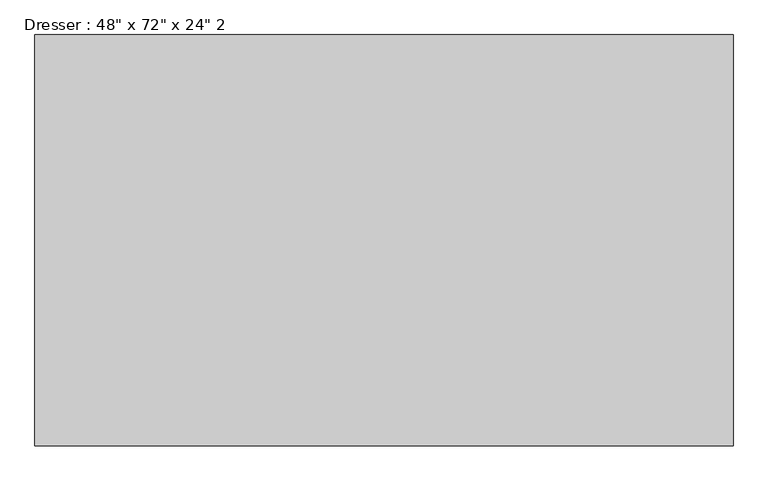
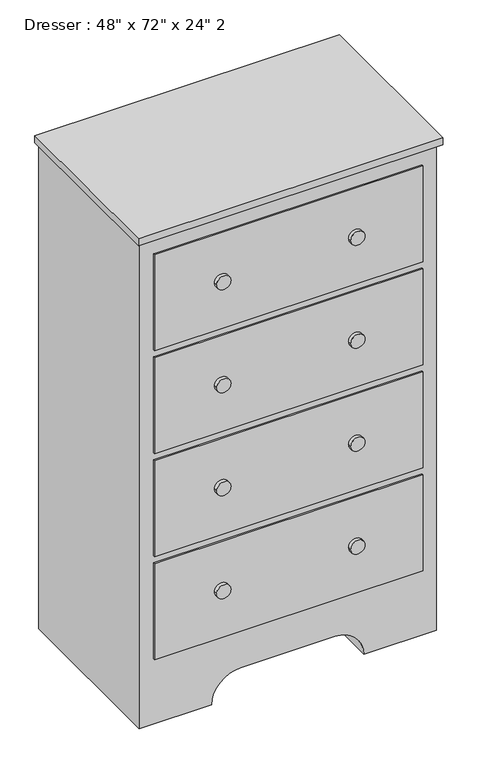
"""IFC4 building model written with IfcOpenShell, lengths in millimetres: furniture geometry."""

from ifc_helpers import new_model, si_unit, point, frame, frame_2d, origin, place, context, project, spatial, polyline, circle_curve, trimmed, segment, composite_curve, outline, extrude, source, transform, mapped, element, save


def furniture_f72bdee3(model_context):
    return source(origin(), model_context, "Body", "SweptSolid", [
        extrude(outline(polyline([(264.2067402, -58.3629541), (264.2067402, -687.0129541), (-802.5932598, -687.0129541), (-802.5932598, -58.3629541), (264.2067402, -58.3629541)])), frame((0.0, 0.0, 1803.4), z_axis=(0.0, 0.0, 1.0), x_axis=(1.0, 0.0, 0.0)), (0.0, 0.0, 1.0), 25.4),
        extrude(outline(composite_curve([segment(polyline([(0.0, 251.5067402), (1803.4, 251.5067402), (1803.4, -789.8932598), (0.0, -789.8932598), (0.0, -535.8932598)]), True, "CONTINUOUS"), segment(trimmed(circle_curve(frame_2d((0.0, -434.2932598)), 101.6), [point((0.0, -535.8932598))], [point((101.6, -434.2932598))], True, "CARTESIAN"), True, "CONTINUOUS"), segment(polyline([(101.6, -434.2932598), (101.6, -104.0932598)]), True, "CONTINUOUS"), segment(trimmed(circle_curve(frame_2d((0.0, -104.0932598)), 101.6), [point((101.6, -104.0932598))], [point((0.0, -2.4932598))], True, "CARTESIAN"), True, "CONTINUOUS"), segment(polyline([(0.0, -2.4932598), (0.0, 251.5067402)]), True, "CONTINUOUS")], self_intersect=False)), frame((0.0, -667.9629541, 0.0), z_axis=(0.0, 1.0, 0.0), x_axis=(0.0, 0.0, 1.0)), (0.0, 0.0, 1.0), 609.6),
        extrude(outline(composite_curve([segment(trimmed(circle_curve(frame_2d((1562.1, -34.2432598)), 25.4), [point((1562.1, -59.6432598))], [point((1562.1, -8.8432598))], False, "CARTESIAN"), True, "CONTINUOUS"), segment(trimmed(circle_curve(frame_2d((1562.1, -34.2432598)), 25.4), [point((1562.1, -8.8432598))], [point((1562.1, -59.6432598))], False, "CARTESIAN"), True, "CONTINUOUS")], self_intersect=False)), frame((0.0, -687.0129541, 0.0), z_axis=(0.0, 1.0, 0.0), x_axis=(0.0, 0.0, 1.0)), (0.0, 0.0, 1.0), 12.7),
        extrude(outline(composite_curve([segment(trimmed(circle_curve(frame_2d((1181.1, -34.2432598)), 25.4), [point((1181.1, -59.6432598))], [point((1181.1, -8.8432598))], False, "CARTESIAN"), True, "CONTINUOUS"), segment(trimmed(circle_curve(frame_2d((1181.1, -34.2432598)), 25.4), [point((1181.1, -8.8432598))], [point((1181.1, -59.6432598))], False, "CARTESIAN"), True, "CONTINUOUS")], self_intersect=False)), frame((0.0, -687.0129541, 0.0), z_axis=(0.0, 1.0, 0.0), x_axis=(0.0, 0.0, 1.0)), (0.0, 0.0, 1.0), 12.7),
        extrude(outline(composite_curve([segment(trimmed(circle_curve(frame_2d((800.1, -34.2432598)), 25.4), [point((800.1, -59.6432598))], [point((800.1, -8.8432598))], False, "CARTESIAN"), True, "CONTINUOUS"), segment(trimmed(circle_curve(frame_2d((800.1, -34.2432598)), 25.4), [point((800.1, -8.8432598))], [point((800.1, -59.6432598))], False, "CARTESIAN"), True, "CONTINUOUS")], self_intersect=False)), frame((0.0, -687.0129541, 0.0), z_axis=(0.0, 1.0, 0.0), x_axis=(0.0, 0.0, 1.0)), (0.0, 0.0, 1.0), 12.7),
        extrude(outline(composite_curve([segment(trimmed(circle_curve(frame_2d((419.1, -34.2432598)), 25.4), [point((419.1, -59.6432598))], [point((419.1, -8.8432598))], False, "CARTESIAN"), True, "CONTINUOUS"), segment(trimmed(circle_curve(frame_2d((419.1, -34.2432598)), 25.4), [point((419.1, -8.8432598))], [point((419.1, -59.6432598))], False, "CARTESIAN"), True, "CONTINUOUS")], self_intersect=False)), frame((0.0, -687.0129541, 0.0), z_axis=(0.0, 1.0, 0.0), x_axis=(0.0, 0.0, 1.0)), (0.0, 0.0, 1.0), 12.7),
        extrude(outline(composite_curve([segment(trimmed(circle_curve(frame_2d((419.1, -504.1432598)), 25.4), [point((419.1, -529.5432598))], [point((419.1, -478.7432598))], False, "CARTESIAN"), True, "CONTINUOUS"), segment(trimmed(circle_curve(frame_2d((419.1, -504.1432598)), 25.4), [point((419.1, -478.7432598))], [point((419.1, -529.5432598))], False, "CARTESIAN"), True, "CONTINUOUS")], self_intersect=False)), frame((0.0, -687.0129541, 0.0), z_axis=(0.0, 1.0, 0.0), x_axis=(0.0, 0.0, 1.0)), (0.0, 0.0, 1.0), 12.7),
        extrude(outline(composite_curve([segment(trimmed(circle_curve(frame_2d((800.1, -504.1432598)), 25.4), [point((800.1, -529.5432598))], [point((800.1, -478.7432598))], False, "CARTESIAN"), True, "CONTINUOUS"), segment(trimmed(circle_curve(frame_2d((800.1, -504.1432598)), 25.4), [point((800.1, -478.7432598))], [point((800.1, -529.5432598))], False, "CARTESIAN"), True, "CONTINUOUS")], self_intersect=False)), frame((0.0, -687.0129541, 0.0), z_axis=(0.0, 1.0, 0.0), x_axis=(0.0, 0.0, 1.0)), (0.0, 0.0, 1.0), 12.7),
        extrude(outline(composite_curve([segment(trimmed(circle_curve(frame_2d((1181.1, -504.1432598)), 25.4), [point((1181.1, -529.5432598))], [point((1181.1, -478.7432598))], False, "CARTESIAN"), True, "CONTINUOUS"), segment(trimmed(circle_curve(frame_2d((1181.1, -504.1432598)), 25.4), [point((1181.1, -478.7432598))], [point((1181.1, -529.5432598))], False, "CARTESIAN"), True, "CONTINUOUS")], self_intersect=False)), frame((0.0, -687.0129541, 0.0), z_axis=(0.0, 1.0, 0.0), x_axis=(0.0, 0.0, 1.0)), (0.0, 0.0, 1.0), 12.7),
        extrude(outline(composite_curve([segment(trimmed(circle_curve(frame_2d((1562.1, -504.1432598)), 25.4), [point((1562.1, -529.5432598))], [point((1562.1, -478.7432598))], False, "CARTESIAN"), True, "CONTINUOUS"), segment(trimmed(circle_curve(frame_2d((1562.1, -504.1432598)), 25.4), [point((1562.1, -478.7432598))], [point((1562.1, -529.5432598))], False, "CARTESIAN"), True, "CONTINUOUS")], self_intersect=False)), frame((0.0, -687.0129541, 0.0), z_axis=(0.0, 1.0, 0.0), x_axis=(0.0, 0.0, 1.0)), (0.0, 0.0, 1.0), 12.7),
        extrude(outline(polyline([(200.7067402, -674.3129541), (-739.0932598, -674.3129541), (-739.0932598, -667.9629541), (200.7067402, -667.9629541), (200.7067402, -674.3129541)])), frame((0.0, 0.0, 1384.3), z_axis=(0.0, 0.0, 1.0), x_axis=(1.0, 0.0, 0.0)), (0.0, 0.0, 1.0), 355.6),
        extrude(outline(polyline([(200.7067402, -674.3129541), (-739.0932598, -674.3129541), (-739.0932598, -667.9629541), (200.7067402, -667.9629541), (200.7067402, -674.3129541)])), frame((0.0, 0.0, 1003.3), z_axis=(0.0, 0.0, 1.0), x_axis=(1.0, 0.0, 0.0)), (0.0, 0.0, 1.0), 355.6),
        extrude(outline(polyline([(200.7067402, -674.3129541), (-739.0932598, -674.3129541), (-739.0932598, -667.9629541), (200.7067402, -667.9629541), (200.7067402, -674.3129541)])), frame((0.0, 0.0, 622.3), z_axis=(0.0, 0.0, 1.0), x_axis=(1.0, 0.0, 0.0)), (0.0, 0.0, 1.0), 355.6),
        extrude(outline(polyline([(200.7067402, -674.3129541), (-739.0932598, -674.3129541), (-739.0932598, -667.9629541), (200.7067402, -667.9629541), (200.7067402, -674.3129541)])), frame((0.0, 0.0, 241.3), z_axis=(0.0, 0.0, 1.0), x_axis=(1.0, 0.0, 0.0)), (0.0, 0.0, 1.0), 355.6),
    ])


if __name__ == "__main__":
    model = new_model("IFC4")
    model_context = context("Model", 3, world=origin())
    ifc_project = project(units=[si_unit("LENGTHUNIT", "METRE", prefix="MILLI")], contexts=[model_context])
    site = spatial("IfcSite", under=ifc_project)
    building = spatial("IfcBuilding", under=site)
    placement = place(None, origin())
    furniture_shape = furniture_f72bdee3(model_context)
    element("IfcFurniture", 1, ObjectType="Dresser : 48\" x 72\" x 24\" 2", at=placement, inside=building, context=model_context, shape_type="MappedRepresentation", body=[
        mapped(furniture_shape, transform((0.0, 0.0, 0.0), x_axis=(1.0, 0.0, 0.0), y_axis=(0.0, 1.0, 0.0), z_axis=(0.0, 0.0, 1.0))),
    ])
    save(model, "model.ifc")

# Revit data of these elements
# Type "Dresser : 48\" x 72\" x 24\" 2"
#   Assembly Code = "E2020200"
#   Depth = 2' - 0"
#   Height = 6' - 0"
#   Width = 3' - 5"
#   Dresser Material = Wood - Teak
#   Drawer Material = Wood - Teak
#   Knob Material = Cherry
#   Default Elevation = 0
# Element 1 (IfcFurniture, "Dresser : 48\" x 72\" x 24\" 2")
#   Materials on its faces: "Laminate, Ivory, Matte", "Cherry", "Wood - Teak"
# Materials
#   "Wood - Teak": class "Wood", colour RGB 145 112 90, transparency 0
#   "Cherry": class "Wood", colour RGB 226 177 128, transparency 0, Description = "Prunus Serotina", Cost = 0
#   "Laminate, Ivory, Matte": class "Plastic", colour RGB 247 247 239, transparency 0, Description = "Plastic Laminate - Ivory, Matte", Cost = 0
